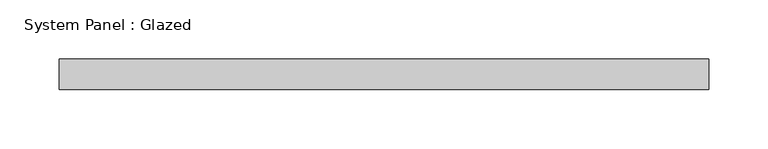
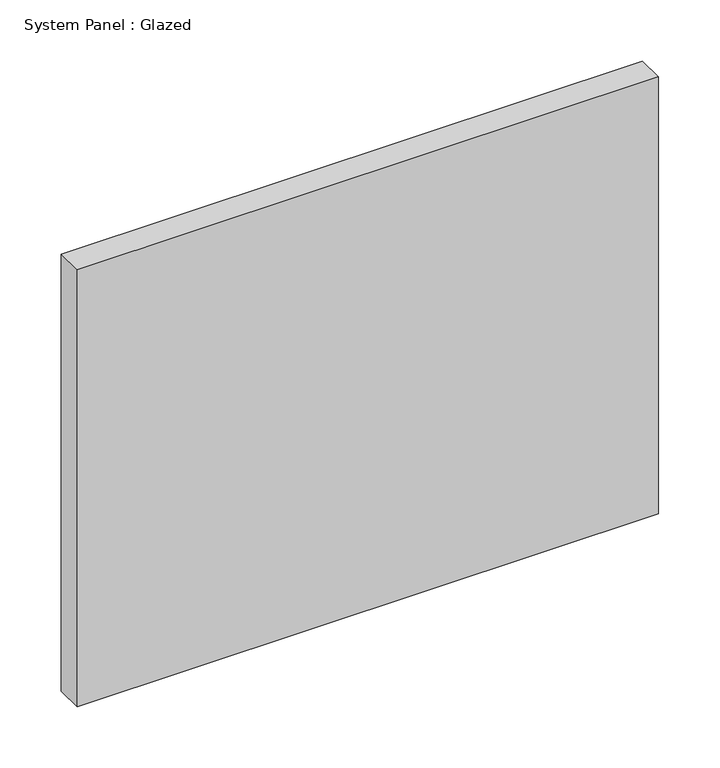
"""IFC4 building model written with IfcOpenShell, lengths in millimetres: plate geometry, System Panel : Glazed."""

from ifc_helpers import new_model, si_unit, origin, origin_with_axes, place, context, project, spatial, polyline, outline, extrude, source, transform, mapped, element, save


def system_panel_glazed_9e7866c3(model_context):
    return source(origin(), model_context, "Body", "SweptSolid", [
        extrude(outline(polyline([(273.05, 19.05), (-273.05, 19.05), (-273.05, 44.45), (273.05, 44.45), (273.05, 19.05)])), origin_with_axes(), (0.0, 0.0, 1.0), 433.9166667),
    ])


if __name__ == "__main__":
    model = new_model("IFC4")
    model_context = context("Model", 3, world=origin())
    ifc_project = project(units=[si_unit("LENGTHUNIT", "METRE", prefix="MILLI")], contexts=[model_context])
    site = spatial("IfcSite", under=ifc_project)
    building = spatial("IfcBuilding", under=site)
    placement = place(None, origin())
    system_panel_glazed_shape = system_panel_glazed_9e7866c3(model_context)
    element("IfcPlate", 1, ObjectType="System Panel : Glazed", at=placement, inside=building, context=model_context, shape_type="MappedRepresentation", body=[
        mapped(system_panel_glazed_shape, transform((0.0, 0.0, 0.0), x_axis=(1.0, 0.0, 0.0), y_axis=(0.0, 1.0, 0.0), z_axis=(0.0, 0.0, 1.0))),
    ])
    save(model, "model.ifc")

# Revit data of these elements
# Type "System Panel : Glazed"
#   Construction Type Id = "GSP4R"
#   Analytic Construction = "1/8 in Pilkington single glazing"
#   Visual Light Transmittance = 0.9
#   Solar Heat Gain Coefficient = 0.86
#   Heat Transfer Coefficient (U) = 1.18115 BTU/(h·ft²·°F)
#   Define Thermal Properties by = 1
# Element 1 (IfcPlate, "System Panel : Glazed")
#   Materials on its faces: "Glass"
# Materials
#   "Glass": class "Glass", colour RGB 0 128 192, transparency 0.75, Description = "Soda Lime Glass", Cost = 0
